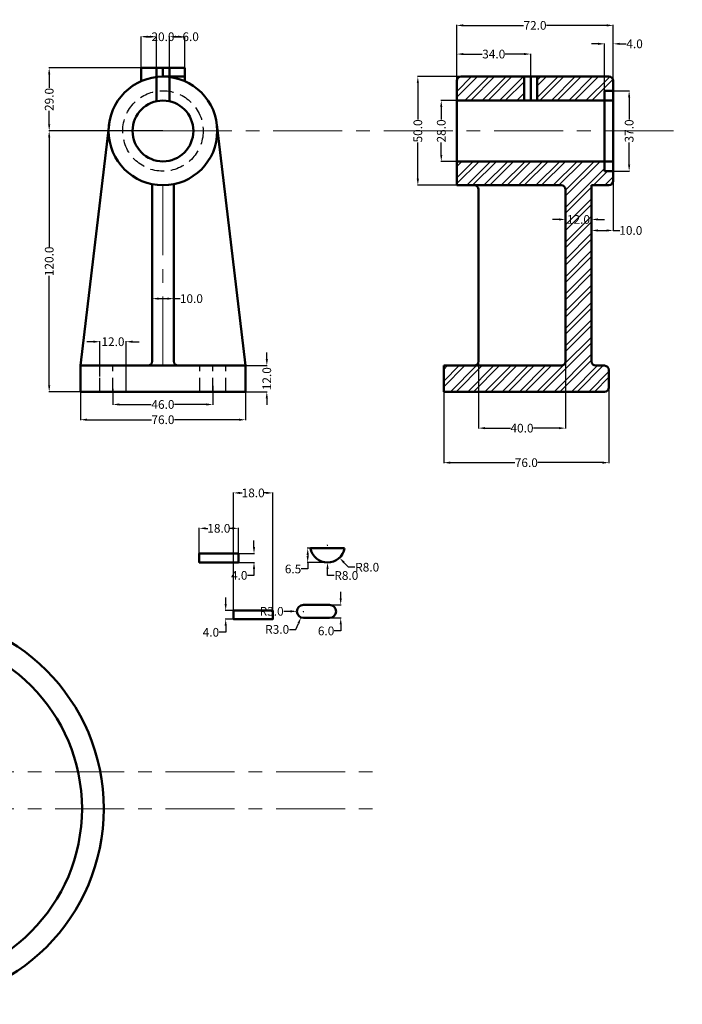
# Model space of a CAD drawing. Units: inches. Extents: x -30 to 602, y 452 to 930.
# Tile 3 of 3: x 297 to 602, y 452 to 905. Entities that reach past the tile are written whole.
import ezdxf

# ---------------------------------------------------------------- set-up
doc = ezdxf.new("R2010")
doc.units = ezdxf.units.IN
doc.header["$MEASUREMENT"] = 0
doc.linetypes.add('CENTER', pattern=[50.8, 31.75, -6.35, 6.35, -6.35])
doc.linetypes.add('HIDDEN', pattern=[9.525, 6.35, -3.175])
for name, color, linetype, lineweight in [('M-CNTR', 1, 'CENTER', 18), ('M-DIMS', 2, 'Continuous', 25), ('M-HATC', 8, 'Continuous', 18), ('M-HIDN', 6, 'HIDDEN', 25), ('M-OUTL', 7, 'Continuous', 50)]:
    doc.layers.add(name, color=color, linetype=linetype, lineweight=lineweight)
doc.styles.get("Standard").update_dxf_attribs({"font": 'arial.ttf'})
doc.dimstyles.get("Standard").update_dxf_attribs({"dimtxt": 4, "dimasz": 3, "dimexe": 0.18, "dimexo": 0.0625, "dimgap": 0.09, "dimtad": 0, "dimtoh": 1, "dimdec": 1, "dimzin": 0, "dimdsep": 46, "dimtxsty": 'Standard', "dimcen": 0.09, "dimadec": 0, "dimazin": 0, "dimtfac": 1, "dimtdec": 1, "dimtofl": 0, "dimtmove": 0, "dimatfit": 3, "dimfxl": 1, "dimtolj": 1, "dimtzin": 0, "dimarcsym": 0})

# ---------------------------------------------------------------- blocks, each defined once
blk = doc.blocks.new('*D16')
at = {"layer": 'Defpoints', "color": 0, "transparency": 16777216}
for p in [(395.82, 745.65), (395.82, 733.65), (410.52, 733.65)]:
    blk.add_point(p, dxfattribs=at)
at = {"layer": 'M-DIMS', "color": 0, "lineweight": -2, "transparency": 16777216}
for p, q in [((410.52, 748.65), (410.52, 751.65)), ((395.88, 745.65), (410.7, 745.65)), ((395.88, 733.65), (410.7, 733.65)), ((410.52, 730.65), (410.52, 727.65))]:
    blk.add_line(p, q, dxfattribs=at)
at = {"layer": 'M-DIMS', "color": 0, "transparency": 16777216}
for points in [[(410.02, 748.65), (411.02, 748.65), (410.52, 745.65)], [(410.02, 730.65), (411.02, 730.65), (410.52, 733.65)]]:
    blk.add_solid(points, dxfattribs=at)
at = {"layer": 'M-DIMS', "color": 0, "transparency": 16777216, "insert": (410.52, 739.65), "char_height": 4, "attachment_point": 5, "rotation": 90}
blk.add_mtext('\\A1;12.0', dxfattribs=at)
blk = doc.blocks.new('*D17')
at = {"layer": 'Defpoints', "color": 0, "transparency": 16777216}
for p in [(367.72, 776.49), (357.72, 770.92), (367.72, 770.92)]:
    blk.add_point(p, dxfattribs=at)
at = {"layer": 'M-DIMS', "color": 0, "lineweight": -2, "transparency": 16777216}
for p, q in [((357.72, 770.98), (357.72, 776.67)), ((360.72, 776.49), (364.72, 776.49)), ((367.72, 770.98), (367.72, 776.67)), ((367.72, 776.49), (370.72, 776.49))]:
    blk.add_line(p, q, dxfattribs=at)
at = {"layer": 'M-DIMS', "color": 0, "transparency": 16777216}
for points in [[(360.72, 776.99), (360.72, 775.99), (357.72, 776.49)], [(364.72, 776.99), (364.72, 775.99), (367.72, 776.49)]]:
    blk.add_solid(points, dxfattribs=at)
at = {"layer": 'M-DIMS', "color": 0, "transparency": 16777216, "insert": (375.81, 776.49), "char_height": 4, "attachment_point": 5}
blk.add_mtext('\\A1;10.0', dxfattribs=at)
blk = doc.blocks.new('*D18')
at = {"layer": 'Defpoints', "color": 0, "transparency": 16777216}
for p in [(345.72, 756.67), (333.72, 740.57), (345.72, 739.65)]:
    blk.add_point(p, dxfattribs=at)
at = {"layer": 'M-DIMS', "color": 0, "lineweight": -2, "transparency": 16777216}
for p, q in [((330.72, 756.67), (327.72, 756.67)), ((333.72, 740.63), (333.72, 756.85)), ((345.72, 739.71), (345.72, 756.85)), ((348.72, 756.67), (351.72, 756.67))]:
    blk.add_line(p, q, dxfattribs=at)
at = {"layer": 'M-DIMS', "color": 0, "transparency": 16777216}
for points in [[(330.72, 757.17), (330.72, 756.17), (333.72, 756.67)], [(348.72, 757.17), (348.72, 756.17), (345.72, 756.67)]]:
    blk.add_solid(points, dxfattribs=at)
at = {"layer": 'M-DIMS', "color": 0, "transparency": 16777216, "insert": (339.72, 756.67), "char_height": 4, "attachment_point": 5}
blk.add_mtext('\\A1;12.0', dxfattribs=at)
blk = doc.blocks.new('*D19')
at = {"layer": 'Defpoints', "color": 0, "transparency": 16777216}
for p in [(339.72, 735.01), (385.72, 736.37), (385.72, 727.79)]:
    blk.add_point(p, dxfattribs=at)
at = {"layer": 'M-DIMS', "color": 0, "lineweight": -2, "transparency": 16777216}
for p, q in [((339.72, 734.94), (339.72, 727.61)), ((385.72, 736.31), (385.72, 727.61)), ((342.72, 727.79), (357.37, 727.79)), ((382.72, 727.79), (368.08, 727.79))]:
    blk.add_line(p, q, dxfattribs=at)
at = {"layer": 'M-DIMS', "color": 0, "transparency": 16777216}
for points in [[(342.72, 728.29), (342.72, 727.29), (339.72, 727.79)], [(382.72, 728.29), (382.72, 727.29), (385.72, 727.79)]]:
    blk.add_solid(points, dxfattribs=at)
at = {"layer": 'M-DIMS', "color": 0, "transparency": 16777216, "insert": (362.72, 727.79), "char_height": 4, "attachment_point": 5}
blk.add_mtext('\\A1;46.0', dxfattribs=at)
blk = doc.blocks.new('*D20')
at = {"layer": 'Defpoints', "color": 0, "transparency": 16777216}
for p in [(324.72, 733.65), (400.72, 733.65), (400.72, 720.77)]:
    blk.add_point(p, dxfattribs=at)
at = {"layer": 'M-DIMS', "color": 0, "lineweight": -2, "transparency": 16777216}
for p, q in [((324.72, 733.59), (324.72, 720.59)), ((400.72, 733.59), (400.72, 720.59)), ((327.72, 720.77), (357.46, 720.77)), ((397.72, 720.77), (367.99, 720.77))]:
    blk.add_line(p, q, dxfattribs=at)
at = {"layer": 'M-DIMS', "color": 0, "transparency": 16777216}
for points in [[(327.72, 721.27), (327.72, 720.27), (324.72, 720.77)], [(397.72, 721.27), (397.72, 720.27), (400.72, 720.77)]]:
    blk.add_solid(points, dxfattribs=at)
at = {"layer": 'M-DIMS', "color": 0, "transparency": 16777216, "insert": (362.72, 720.77), "char_height": 4, "attachment_point": 5}
blk.add_mtext('\\A1;76.0', dxfattribs=at)
blk = doc.blocks.new('*D21')
at = {"layer": 'Defpoints', "color": 0, "transparency": 16777216}
for p in [(569.95, 902.22), (497.95, 865.23), (569.95, 860.94)]:
    blk.add_point(p, dxfattribs=at)
at = {"layer": 'M-DIMS', "color": 0, "lineweight": -2, "transparency": 16777216}
for p, q in [((497.95, 865.29), (497.95, 902.4)), ((500.95, 902.22), (528.69, 902.22)), ((566.95, 902.22), (539.22, 902.22)), ((569.95, 861), (569.95, 902.4))]:
    blk.add_line(p, q, dxfattribs=at)
at = {"layer": 'M-DIMS', "color": 0, "transparency": 16777216}
for points in [[(500.95, 902.72), (500.95, 901.72), (497.95, 902.22)], [(566.95, 902.72), (566.95, 901.72), (569.95, 902.22)]]:
    blk.add_solid(points, dxfattribs=at)
at = {"layer": 'M-DIMS', "color": 0, "transparency": 16777216, "insert": (533.95, 902.22), "char_height": 4, "attachment_point": 5}
blk.add_mtext('\\A1;72.0', dxfattribs=at)
blk = doc.blocks.new('*D22')
at = {"layer": 'Defpoints', "color": 0, "transparency": 16777216}
for p in [(497.95, 889.02), (497.95, 873.15), (531.95, 873.15)]:
    blk.add_point(p, dxfattribs=at)
at = {"layer": 'M-DIMS', "color": 0, "lineweight": -2, "transparency": 16777216}
for p, q in [((497.95, 873.21), (497.95, 889.2)), ((500.95, 889.02), (509.68, 889.02)), ((528.95, 889.02), (520.23, 889.02)), ((531.95, 873.21), (531.95, 889.2))]:
    blk.add_line(p, q, dxfattribs=at)
at = {"layer": 'M-DIMS', "color": 0, "transparency": 16777216}
for points in [[(500.95, 889.52), (500.95, 888.52), (497.95, 889.02)], [(528.95, 889.52), (528.95, 888.52), (531.95, 889.02)]]:
    blk.add_solid(points, dxfattribs=at)
at = {"layer": 'M-DIMS', "color": 0, "transparency": 16777216, "insert": (514.95, 889.02), "char_height": 4, "attachment_point": 5}
blk.add_mtext('\\A1;34.0', dxfattribs=at)
blk = doc.blocks.new('*D23')
at = {"layer": 'Defpoints', "color": 0, "transparency": 16777216}
for p in [(569.95, 893.73), (569.95, 861.83), (565.95, 860.76)]:
    blk.add_point(p, dxfattribs=at)
at = {"layer": 'M-DIMS', "color": 0, "lineweight": -2, "transparency": 16777216}
for p, q in [((562.95, 893.73), (559.95, 893.73)), ((565.95, 860.82), (565.95, 893.91)), ((569.95, 861.89), (569.95, 893.91)), ((572.95, 893.73), (575.95, 893.73))]:
    blk.add_line(p, q, dxfattribs=at)
at = {"layer": 'M-DIMS', "color": 0, "transparency": 16777216}
for points in [[(562.95, 894.23), (562.95, 893.23), (565.95, 893.73)], [(572.95, 894.23), (572.95, 893.23), (569.95, 893.73)]]:
    blk.add_solid(points, dxfattribs=at)
at = {"layer": 'M-DIMS', "color": 0, "transparency": 16777216, "insert": (579.76, 893.73), "char_height": 4, "attachment_point": 5}
blk.add_mtext('\\A1;4.0', dxfattribs=at)
blk = doc.blocks.new('*D24')
at = {"layer": 'Defpoints', "color": 0, "transparency": 16777216}
for p in [(569.95, 872.15), (569.95, 835.15), (577.26, 835.15)]:
    blk.add_point(p, dxfattribs=at)
at = {"layer": 'M-DIMS', "color": 0, "lineweight": -2, "transparency": 16777216}
for p, q in [((570.02, 872.15), (577.44, 872.15)), ((577.26, 869.15), (577.26, 858.93)), ((577.26, 838.15), (577.26, 848.37)), ((570.02, 835.15), (577.44, 835.15))]:
    blk.add_line(p, q, dxfattribs=at)
at = {"layer": 'M-DIMS', "color": 0, "transparency": 16777216}
for points in [[(576.76, 869.15), (577.76, 869.15), (577.26, 872.15)], [(576.76, 838.15), (577.76, 838.15), (577.26, 835.15)]]:
    blk.add_solid(points, dxfattribs=at)
at = {"layer": 'M-DIMS', "color": 0, "transparency": 16777216, "insert": (577.26, 853.65), "char_height": 4, "attachment_point": 5, "rotation": 90}
blk.add_mtext('\\A1;37.0', dxfattribs=at)
blk = doc.blocks.new('*D25')
at = {"layer": 'Defpoints', "color": 0, "transparency": 16777216}
for p in [(501.37, 867.65), (490.8, 839.65), (501.37, 839.65)]:
    blk.add_point(p, dxfattribs=at)
at = {"layer": 'M-DIMS', "color": 0, "lineweight": -2, "transparency": 16777216}
for p, q in [((501.3, 867.65), (490.62, 867.65)), ((490.8, 864.65), (490.8, 858.96)), ((490.8, 842.65), (490.8, 848.34)), ((501.3, 839.65), (490.62, 839.65))]:
    blk.add_line(p, q, dxfattribs=at)
at = {"layer": 'M-DIMS', "color": 0, "transparency": 16777216}
for points in [[(490.3, 864.65), (491.3, 864.65), (490.8, 867.65)], [(490.3, 842.65), (491.3, 842.65), (490.8, 839.65)]]:
    blk.add_solid(points, dxfattribs=at)
at = {"layer": 'M-DIMS', "color": 0, "transparency": 16777216, "insert": (490.8, 853.65), "char_height": 4, "attachment_point": 5, "rotation": 90}
blk.add_mtext('\\A1;28.0', dxfattribs=at)
blk = doc.blocks.new('*D26')
at = {"layer": 'Defpoints', "color": 0, "transparency": 16777216}
for p in [(502.42, 878.65), (480.02, 828.65), (499.89, 828.65)]:
    blk.add_point(p, dxfattribs=at)
at = {"layer": 'M-DIMS', "color": 0, "lineweight": -2, "transparency": 16777216}
for p, q in [((502.36, 878.65), (479.84, 878.65)), ((480.02, 875.65), (480.02, 858.93)), ((480.02, 831.65), (480.02, 848.37)), ((499.82, 828.65), (479.84, 828.65))]:
    blk.add_line(p, q, dxfattribs=at)
at = {"layer": 'M-DIMS', "color": 0, "transparency": 16777216}
for points in [[(479.52, 875.65), (480.52, 875.65), (480.02, 878.65)], [(479.52, 831.65), (480.52, 831.65), (480.02, 828.65)]]:
    blk.add_solid(points, dxfattribs=at)
at = {"layer": 'M-DIMS', "color": 0, "transparency": 16777216, "insert": (480.02, 853.65), "char_height": 4, "attachment_point": 5, "rotation": 90}
blk.add_mtext('\\A1;50.0', dxfattribs=at)
blk = doc.blocks.new('*D27')
at = {"layer": 'Defpoints', "color": 0, "transparency": 16777216}
for p in [(547.95, 812.93), (559.95, 812.93), (559.95, 811.58)]:
    blk.add_point(p, dxfattribs=at)
at = {"layer": 'M-DIMS', "color": 0, "lineweight": -2, "transparency": 16777216}
for p, q in [((544.95, 812.93), (541.95, 812.93)), ((547.95, 812.99), (547.95, 813.11)), ((559.95, 811.64), (559.95, 813.11)), ((562.95, 812.93), (565.95, 812.93))]:
    blk.add_line(p, q, dxfattribs=at)
at = {"layer": 'M-DIMS', "color": 0, "transparency": 16777216}
for points in [[(544.95, 813.43), (544.95, 812.43), (547.95, 812.93)], [(562.95, 813.43), (562.95, 812.43), (559.95, 812.93)]]:
    blk.add_solid(points, dxfattribs=at)
at = {"layer": 'M-DIMS', "color": 0, "transparency": 16777216, "insert": (553.95, 812.93), "char_height": 4, "attachment_point": 5}
blk.add_mtext('\\A1;12.0', dxfattribs=at)
blk = doc.blocks.new('*D28')
at = {"layer": 'Defpoints', "color": 0, "transparency": 16777216}
for p in [(569.95, 835.15), (559.95, 823.74), (569.95, 807.86)]:
    blk.add_point(p, dxfattribs=at)
at = {"layer": 'M-DIMS', "color": 0, "lineweight": -2, "transparency": 16777216}
for p, q in [((569.95, 835.09), (569.95, 807.68)), ((559.95, 823.67), (559.95, 807.68)), ((562.95, 807.86), (566.95, 807.86)), ((569.95, 807.86), (572.95, 807.86))]:
    blk.add_line(p, q, dxfattribs=at)
at = {"layer": 'M-DIMS', "color": 0, "transparency": 16777216}
for points in [[(562.95, 808.36), (562.95, 807.36), (559.95, 807.86)], [(566.95, 808.36), (566.95, 807.36), (569.95, 807.86)]]:
    blk.add_solid(points, dxfattribs=at)
at = {"layer": 'M-DIMS', "color": 0, "transparency": 16777216, "insert": (578.04, 807.86), "char_height": 4, "attachment_point": 5}
blk.add_mtext('\\A1;10.0', dxfattribs=at)
blk = doc.blocks.new('*D29')
at = {"layer": 'Defpoints', "color": 0, "transparency": 16777216}
for p in [(491.95, 739.65), (567.95, 741.21), (567.95, 701.02)]:
    blk.add_point(p, dxfattribs=at)
at = {"layer": 'M-DIMS', "color": 0, "lineweight": -2, "transparency": 16777216}
for p, q in [((491.95, 739.59), (491.95, 700.84)), ((567.95, 741.15), (567.95, 700.84)), ((494.95, 701.02), (524.69, 701.02)), ((564.95, 701.02), (535.22, 701.02))]:
    blk.add_line(p, q, dxfattribs=at)
at = {"layer": 'M-DIMS', "color": 0, "transparency": 16777216}
for points in [[(494.95, 701.52), (494.95, 700.52), (491.95, 701.02)], [(564.95, 701.52), (564.95, 700.52), (567.95, 701.02)]]:
    blk.add_solid(points, dxfattribs=at)
at = {"layer": 'M-DIMS', "color": 0, "transparency": 16777216, "insert": (529.95, 701.02), "char_height": 4, "attachment_point": 5}
blk.add_mtext('\\A1;76.0', dxfattribs=at)
blk = doc.blocks.new('*D30')
at = {"layer": 'Defpoints', "color": 0, "transparency": 16777216}
for p in [(507.95, 764.86), (547.95, 764.86), (547.95, 716.9)]:
    blk.add_point(p, dxfattribs=at)
at = {"layer": 'M-DIMS', "color": 0, "lineweight": -2, "transparency": 16777216}
for p, q in [((507.95, 764.79), (507.95, 716.72)), ((547.95, 764.79), (547.95, 716.72)), ((510.95, 716.9), (522.59, 716.9)), ((544.95, 716.9), (533.31, 716.9))]:
    blk.add_line(p, q, dxfattribs=at)
at = {"layer": 'M-DIMS', "color": 0, "transparency": 16777216}
for points in [[(510.95, 717.4), (510.95, 716.4), (507.95, 716.9)], [(544.95, 717.4), (544.95, 716.4), (547.95, 716.9)]]:
    blk.add_solid(points, dxfattribs=at)
at = {"layer": 'M-DIMS', "color": 0, "transparency": 16777216, "insert": (527.95, 716.9), "char_height": 4, "attachment_point": 5}
blk.add_mtext('\\A1;40.0', dxfattribs=at)
blk = doc.blocks.new('*D44')
at = {"layer": 'Defpoints', "color": 0, "transparency": 16777216}
for p in [(397.44, 670.8), (379.44, 657.76), (397.44, 657.15)]:
    blk.add_point(p, dxfattribs=at)
at = {"layer": 'M-DIMS', "color": 0, "lineweight": -2, "transparency": 16777216}
for p, q in [((379.44, 657.82), (379.44, 670.98)), ((382.44, 670.8), (383.35, 670.8)), ((394.44, 670.8), (393.53, 670.8)), ((397.44, 657.22), (397.44, 670.98))]:
    blk.add_line(p, q, dxfattribs=at)
at = {"layer": 'M-DIMS', "color": 0, "transparency": 16777216}
for points in [[(382.44, 671.3), (382.44, 670.3), (379.44, 670.8)], [(394.44, 671.3), (394.44, 670.3), (397.44, 670.8)]]:
    blk.add_solid(points, dxfattribs=at)
at = {"layer": 'M-DIMS', "color": 0, "transparency": 16777216, "insert": (388.44, 670.8), "char_height": 4, "attachment_point": 5}
blk.add_mtext('\\A1;18.0', dxfattribs=at)
blk = doc.blocks.new('*D45')
at = {"layer": 'Defpoints', "color": 0, "transparency": 16777216}
for p in [(397.44, 659.15), (397.44, 655.15), (404.62, 655.15)]:
    blk.add_point(p, dxfattribs=at)
at = {"layer": 'M-DIMS', "color": 0, "lineweight": -2, "transparency": 16777216}
for p, q in [((404.62, 662.15), (404.62, 665.15)), ((397.5, 659.15), (404.8, 659.15)), ((397.5, 655.15), (404.8, 655.15)), ((404.62, 649.15), (401.62, 649.15)), ((404.62, 652.15), (404.62, 649.15))]:
    blk.add_line(p, q, dxfattribs=at)
at = {"layer": 'M-DIMS', "color": 0, "transparency": 16777216}
for points in [[(404.12, 662.15), (405.12, 662.15), (404.62, 659.15)], [(404.12, 652.15), (405.12, 652.15), (404.62, 655.15)]]:
    blk.add_solid(points, dxfattribs=at)
at = {"layer": 'M-DIMS', "color": 0, "transparency": 16777216, "insert": (397.81, 649.15), "char_height": 4, "attachment_point": 5}
blk.add_mtext('\\A1;4.0', dxfattribs=at)
blk = doc.blocks.new('*D46')
at = {"layer": 'Defpoints', "color": 0, "transparency": 16777216}
for p in [(438.46, 663.1), (443.95, 657.28)]:
    blk.add_point(p, dxfattribs=at)
at = {"layer": 'M-DIMS', "color": 0, "lineweight": -2, "transparency": 16777216}
for p, q in [((438.37, 663.1), (438.55, 663.1)), ((438.46, 663.01), (438.46, 663.19)), ((448.07, 652.92), (446.01, 655.1)), ((451.07, 652.92), (448.07, 652.92))]:
    blk.add_line(p, q, dxfattribs=at)
at = {"layer": 'M-DIMS', "color": 0, "transparency": 16777216}
blk.add_solid([(446.37, 655.44), (445.65, 654.76), (443.95, 657.28)], dxfattribs=at)
at = {"layer": 'M-DIMS', "color": 0, "transparency": 16777216, "insert": (456.71, 652.92), "char_height": 4, "attachment_point": 5}
blk.add_mtext('\\A1;R8.0', dxfattribs=at)
blk = doc.blocks.new('*D47')
at = {"layer": 'Defpoints', "color": 0, "transparency": 16777216}
for p in [(438.46, 661.6), (429.34, 655.1), (438.46, 655.1)]:
    blk.add_point(p, dxfattribs=at)
at = {"layer": 'M-DIMS', "color": 0, "lineweight": -2, "transparency": 16777216}
for p, q in [((438.4, 661.6), (429.16, 661.6)), ((429.34, 658.6), (429.34, 658.1)), ((438.4, 655.1), (429.16, 655.1)), ((429.34, 655.1), (429.34, 652.1)), ((429.34, 652.1), (426.34, 652.1))]:
    blk.add_line(p, q, dxfattribs=at)
at = {"layer": 'M-DIMS', "color": 0, "transparency": 16777216}
for points in [[(428.84, 658.6), (429.84, 658.6), (429.34, 661.6)], [(428.84, 658.1), (429.84, 658.1), (429.34, 655.1)]]:
    blk.add_solid(points, dxfattribs=at)
at = {"layer": 'M-DIMS', "color": 0, "transparency": 16777216, "insert": (422.59, 652.1), "char_height": 4, "attachment_point": 5}
blk.add_mtext('\\A1;6.5', dxfattribs=at)
blk = doc.blocks.new('*D48')
at = {"layer": 'Defpoints', "color": 0, "transparency": 16777216}
for p in [(395.24, 632.97), (391.59, 628.97), (395.24, 628.97)]:
    blk.add_point(p, dxfattribs=at)
at = {"layer": 'M-DIMS', "color": 0, "lineweight": -2, "transparency": 16777216}
for p, q in [((391.59, 635.97), (391.59, 638.97)), ((395.17, 632.97), (391.41, 632.97)), ((395.17, 628.97), (391.41, 628.97)), ((391.59, 625.97), (391.59, 622.97)), ((391.59, 622.97), (388.59, 622.97))]:
    blk.add_line(p, q, dxfattribs=at)
at = {"layer": 'M-DIMS', "color": 0, "transparency": 16777216}
for points in [[(391.09, 635.97), (392.09, 635.97), (391.59, 632.97)], [(391.09, 625.97), (392.09, 625.97), (391.59, 628.97)]]:
    blk.add_solid(points, dxfattribs=at)
at = {"layer": 'M-DIMS', "color": 0, "transparency": 16777216, "insert": (384.79, 622.97), "char_height": 4, "attachment_point": 5}
blk.add_mtext('\\A1;4.0', dxfattribs=at)
blk = doc.blocks.new('*D49')
at = {"layer": 'Defpoints', "color": 0, "transparency": 16777216}
for p in [(433.07, 635.59), (433.07, 629.59), (444.53, 629.59)]:
    blk.add_point(p, dxfattribs=at)
at = {"layer": 'M-DIMS', "color": 0, "lineweight": -2, "transparency": 16777216}
for p, q in [((444.53, 638.59), (444.53, 641.59)), ((433.13, 635.59), (444.71, 635.59)), ((433.13, 629.59), (444.71, 629.59)), ((444.53, 626.59), (444.53, 623.59)), ((444.53, 623.59), (441.53, 623.59))]:
    blk.add_line(p, q, dxfattribs=at)
at = {"layer": 'M-DIMS', "color": 0, "transparency": 16777216}
for points in [[(444.03, 638.59), (445.03, 638.59), (444.53, 635.59)], [(444.03, 626.59), (445.03, 626.59), (444.53, 629.59)]]:
    blk.add_solid(points, dxfattribs=at)
at = {"layer": 'M-DIMS', "color": 0, "transparency": 16777216, "insert": (437.79, 623.59), "char_height": 4, "attachment_point": 5}
blk.add_mtext('\\A1;6.0', dxfattribs=at)
blk = doc.blocks.new('*D50')
at = {"layer": 'Defpoints', "color": 0, "transparency": 16777216}
for p in [(426.24, 629.83), (427.39, 632.59)]:
    blk.add_point(p, dxfattribs=at)
at = {"layer": 'M-DIMS', "color": 0, "lineweight": -2, "transparency": 16777216}
for p, q in [((427.3, 632.59), (427.48, 632.59)), ((427.39, 632.5), (427.39, 632.68)), ((423.92, 624.29), (425.08, 627.06)), ((420.92, 624.29), (423.92, 624.29))]:
    blk.add_line(p, q, dxfattribs=at)
at = {"layer": 'M-DIMS', "color": 0, "transparency": 16777216}
blk.add_solid([(424.62, 627.25), (425.54, 626.87), (426.24, 629.83)], dxfattribs=at)
at = {"layer": 'M-DIMS', "color": 0, "transparency": 16777216, "insert": (415.29, 624.29), "char_height": 4, "attachment_point": 5}
blk.add_mtext('\\A1;R3.0', dxfattribs=at)
blk = doc.blocks.new('*D58')
at = {"layer": 'Defpoints', "color": 0, "transparency": 16777216}
for p in [(310.37, 853.65), (362.72, 853.65), (324.72, 733.65)]:
    blk.add_point(p, dxfattribs=at)
at = {"layer": 'M-DIMS', "color": 0, "lineweight": -2, "transparency": 16777216}
for p, q in [((362.66, 853.65), (310.19, 853.65)), ((310.37, 850.65), (310.37, 800.29)), ((310.37, 736.65), (310.37, 787.01)), ((324.66, 733.65), (310.19, 733.65))]:
    blk.add_line(p, q, dxfattribs=at)
at = {"layer": 'M-DIMS', "color": 0, "transparency": 16777216}
for points in [[(309.87, 850.65), (310.87, 850.65), (310.37, 853.65)], [(309.87, 736.65), (310.87, 736.65), (310.37, 733.65)]]:
    blk.add_solid(points, dxfattribs=at)
at = {"layer": 'M-DIMS', "color": 0, "transparency": 16777216, "insert": (310.37, 793.65), "char_height": 4, "attachment_point": 5, "rotation": 90}
blk.add_mtext('\\A1;120.0', dxfattribs=at)
blk = doc.blocks.new('*D59')
at = {"layer": 'Defpoints', "color": 0, "transparency": 16777216}
for p in [(310.37, 882.65), (352.72, 882.65), (362.72, 853.65)]:
    blk.add_point(p, dxfattribs=at)
at = {"layer": 'M-DIMS', "color": 0, "lineweight": -2, "transparency": 16777216}
for p, q in [((352.66, 882.65), (310.19, 882.65)), ((310.37, 879.65), (310.37, 873.46)), ((310.37, 856.65), (310.37, 862.84)), ((362.66, 853.65), (310.19, 853.65))]:
    blk.add_line(p, q, dxfattribs=at)
at = {"layer": 'M-DIMS', "color": 0, "transparency": 16777216}
for points in [[(309.87, 879.65), (310.87, 879.65), (310.37, 882.65)], [(309.87, 856.65), (310.87, 856.65), (310.37, 853.65)]]:
    blk.add_solid(points, dxfattribs=at)
at = {"layer": 'M-DIMS', "color": 0, "transparency": 16777216, "insert": (310.37, 868.15), "char_height": 4, "attachment_point": 5, "rotation": 90}
blk.add_mtext('\\A1;29.0', dxfattribs=at)
blk = doc.blocks.new('*D60')
at = {"layer": 'Defpoints', "color": 0, "transparency": 16777216}
for p in [(372.72, 897), (352.72, 882.65), (372.72, 882.65)]:
    blk.add_point(p, dxfattribs=at)
at = {"layer": 'M-DIMS', "color": 0, "lineweight": -2, "transparency": 16777216}
for p, q in [((352.72, 882.71), (352.72, 897.18)), ((372.72, 882.71), (372.72, 897.18)), ((355.72, 897), (357.41, 897)), ((369.72, 897), (368.04, 897))]:
    blk.add_line(p, q, dxfattribs=at)
at = {"layer": 'M-DIMS', "color": 0, "transparency": 16777216}
for points in [[(355.72, 897.5), (355.72, 896.5), (352.72, 897)], [(369.72, 897.5), (369.72, 896.5), (372.72, 897)]]:
    blk.add_solid(points, dxfattribs=at)
at = {"layer": 'M-DIMS', "color": 0, "transparency": 16777216, "insert": (362.72, 897), "char_height": 4, "attachment_point": 5}
blk.add_mtext('\\A1;20.0', dxfattribs=at)
blk = doc.blocks.new('*D61')
at = {"layer": 'Defpoints', "color": 0, "transparency": 16777216}
for p in [(365.72, 897), (359.72, 882.65), (365.72, 882.65)]:
    blk.add_point(p, dxfattribs=at)
at = {"layer": 'M-DIMS', "color": 0, "lineweight": -2, "transparency": 16777216}
for p, q in [((359.72, 882.71), (359.72, 897.18)), ((365.72, 882.71), (365.72, 897.18)), ((356.72, 897), (353.72, 897)), ((368.72, 897), (371.72, 897))]:
    blk.add_line(p, q, dxfattribs=at)
at = {"layer": 'M-DIMS', "color": 0, "transparency": 16777216}
for points in [[(356.72, 897.5), (356.72, 896.5), (359.72, 897)], [(368.72, 897.5), (368.72, 896.5), (365.72, 897)]]:
    blk.add_solid(points, dxfattribs=at)
at = {"layer": 'M-DIMS', "color": 0, "transparency": 16777216, "insert": (375.46, 897), "char_height": 4, "attachment_point": 5}
blk.add_mtext('\\A1;6.0', dxfattribs=at)
blk = doc.blocks.new('*D62')
at = {"layer": 'Defpoints', "color": 0, "transparency": 16777216}
for p in [(413.237044, 687.097154), (395.237044, 632.969264), (413.237044, 632.969264)]:
    blk.add_point(p, dxfattribs=at)
at = {"layer": 'M-DIMS', "color": 0, "lineweight": -2, "transparency": 16777216}
for p, q in [((395.237044, 633.031764), (395.237044, 687.277154)), ((398.237044, 687.097154), (399.147044, 687.097154)), ((410.237044, 687.097154), (409.327044, 687.097154)), ((413.237044, 633.031764), (413.237044, 687.277154))]:
    blk.add_line(p, q, dxfattribs=at)
at = {"layer": 'M-DIMS', "color": 0, "transparency": 16777216}
for points in [[(398.237044, 687.597154), (398.237044, 686.597154), (395.237044, 687.097154)], [(410.237044, 687.597154), (410.237044, 686.597154), (413.237044, 687.097154)]]:
    blk.add_solid(points, dxfattribs=at)
at = {"layer": 'M-DIMS', "color": 0, "transparency": 16777216, "insert": (404.237044, 687.097154), "char_height": 4, "attachment_point": 5}
blk.add_mtext('\\A1;18.0', dxfattribs=at)
blk = doc.blocks.new('*D68')
at = {"layer": 'Defpoints', "color": 0, "transparency": 16777216}
for p in [(438.46, 663.1), (438.46, 655.1)]:
    blk.add_point(p, dxfattribs=at)
at = {"layer": 'M-DIMS', "color": 0, "lineweight": -2, "transparency": 16777216}
for p, q in [((438.37, 663.1), (438.55, 663.1)), ((438.46, 663.01), (438.46, 663.19)), ((438.46, 649.1), (438.46, 652.1)), ((441.46, 649.1), (438.46, 649.1))]:
    blk.add_line(p, q, dxfattribs=at)
at = {"layer": 'M-DIMS', "color": 0, "transparency": 16777216}
blk.add_solid([(438.96, 652.1), (437.96, 652.1), (438.46, 655.1)], dxfattribs=at)
at = {"layer": 'M-DIMS', "color": 0, "transparency": 16777216, "insert": (447.1, 649.1), "char_height": 4, "attachment_point": 5}
blk.add_mtext('\\A1;R8.0', dxfattribs=at)
blk = doc.blocks.new('*D69')
at = {"layer": 'Defpoints', "color": 0, "transparency": 16777216}
for p in [(424.39, 632.6), (427.39, 632.59)]:
    blk.add_point(p, dxfattribs=at)
at = {"layer": 'M-DIMS', "color": 0, "lineweight": -2, "transparency": 16777216}
for p, q in [((418.39, 632.61), (421.39, 632.61)), ((427.3, 632.59), (427.48, 632.59)), ((427.39, 632.5), (427.39, 632.68))]:
    blk.add_line(p, q, dxfattribs=at)
at = {"layer": 'M-DIMS', "color": 0, "transparency": 16777216}
blk.add_solid([(421.39, 633.11), (421.39, 632.11), (424.39, 632.6)], dxfattribs=at)
at = {"layer": 'M-DIMS', "color": 0, "transparency": 16777216, "insert": (412.75, 632.61), "char_height": 4, "attachment_point": 5}
blk.add_mtext('\\A1;R3.0', dxfattribs=at)

msp = doc.modelspace()

# ---------------------------------------------------------------- hatches: boundary and pattern name
at = {"layer": 'M-HATC'}
h = msp.add_hatch(dxfattribs=at)
h.set_pattern_fill('ANSI32', color=256, scale=15)
h.paths.add_polyline_path([(528.95, 878.65), (499.95, 878.65, 0.414214), (497.95, 876.65), (497.95, 867.65), (528.95, 867.65)])
h.paths.add_polyline_path([(569.95, 876.65, 0.414214), (567.95, 878.65), (534.95, 878.65), (534.95, 867.65), (565.95, 867.65), (565.95, 872.15), (569.95, 872.15)])
h.paths.add_polyline_path([(559.95, 828.65), (567.95, 828.65, 0.414214), (569.95, 830.65), (569.95, 835.15), (565.95, 835.15), (565.95, 839.65), (497.95, 839.65), (497.95, 828.65), (545.95, 828.65, -0.414214), (547.95, 826.65), (547.95, 747.65, -0.414214), (545.95, 745.65), (491.95, 745.65), (491.95, 733.65), (565.95, 733.65, 0.414214), (567.95, 735.65), (567.95, 743.65, 0.414214), (565.95, 745.65), (561.95, 745.65, -0.414214), (559.95, 747.65)])

# ---------------------------------------------------------------- linework, layer by layer
at = {"layer": 'M-CNTR'}
for p, q in [((362.72, 853.65), (601.73, 853.65)), ((362.72, 745.65), (362.72, 828.65)), ((59.17, 558.79), (462.28, 558.79)), ((59.17, 541.79), (462.28, 541.79))]:
    msp.add_line(p, q, dxfattribs=at)
at = {"layer": 'M-HIDN'}
for p, q in [((333.72, 733.65), (333.72, 745.65)), ((339.72, 733.65), (339.72, 745.65)), ((345.72, 733.65), (345.72, 745.65)), ((379.72, 733.65), (379.72, 745.65)), ((385.72, 733.65), (385.72, 745.65)), ((391.72, 733.65), (391.72, 745.65))]:
    msp.add_line(p, q, dxfattribs=at)
msp.add_circle((362.72, 853.65), 18.5, dxfattribs=at)
at = {"layer": 'M-OUTL'}
for p, q in [((352.72, 882.65), (372.72, 882.65)), ((352.72, 876.56), (352.72, 882.65)), ((359.72, 867.33), (359.72, 882.65)), ((362.72, 878.65), (362.72, 882.65)), ((365.72, 867.33), (365.72, 882.65)), ((372.72, 876.56), (372.72, 882.65)), ((362.72, 878.65), (372.72, 878.65)), ((497.95, 876.65), (497.95, 828.65)), ((499.95, 878.65), (567.95, 878.65)), ((528.95, 878.65), (528.95, 867.65)), ((531.95, 878.65), (531.95, 867.65)), ((534.95, 878.65), (534.95, 867.65)), ((569.95, 876.65), (569.95, 830.65)), ((565.95, 872.15), (569.95, 872.15)), ((565.95, 872.15), (565.95, 835.15)), ((497.95, 867.65), (569.95, 867.65)), ((337.9, 856.6), (324.72, 745.65)), ((387.55, 856.6), (400.72, 745.65)), ((497.95, 839.65), (569.95, 839.65)), ((565.95, 835.15), (569.95, 835.15)), ((357.72, 747.65), (357.72, 829.16)), ((367.72, 747.65), (367.72, 829.16)), ((497.95, 828.65), (545.95, 828.65)), ((507.95, 826.65), (507.95, 747.65)), ((547.95, 826.65), (547.95, 747.65)), ((559.95, 828.65), (559.95, 747.65)), ((559.95, 828.65), (567.95, 828.65)), ((400.72, 745.65), (324.72, 745.65)), ((324.72, 745.65), (324.72, 733.65)), ((400.72, 733.65), (400.72, 745.65)), ((491.95, 745.65), (545.95, 745.65)), ((491.95, 733.65), (491.95, 745.65)), ((561.95, 745.65), (565.95, 745.65)), ((567.95, 743.65), (567.95, 735.65)), ((324.72, 733.65), (400.72, 733.65)), ((565.95, 733.65), (491.95, 733.65)), ((446.32, 661.6), (430.6, 661.6))]:
    msp.add_line(p, q, dxfattribs=at)
for points in [[(379.44, 659.15), (397.44, 659.15), (397.44, 655.15), (379.44, 655.15)], [(395.24, 632.97), (413.24, 632.97), (413.24, 628.97), (395.24, 628.97)]]:
    msp.add_lwpolyline(points, close=True, dxfattribs=at)
for points in [[(427.39, 635.59), (439.39, 635.59)], [(439.39, 629.59), (427.39, 629.59)]]:
    msp.add_lwpolyline(points, dxfattribs=at)
for centre, radius in [((362.72, 853.65), 25), ((362.72, 853.65), 14), ((245.47, 541.79), 90), ((245.47, 541.79), 80)]:
    msp.add_circle(centre, radius, dxfattribs=at)
for centre, radius, start, end in [((499.95, 876.65), 2, 90, 180), ((567.95, 876.65), 2, 0, 90), ((567.95, 830.65), 2, 270, 0), ((505.95, 826.65), 2, 0, 90), ((545.95, 826.65), 2, 0, 90), ((355.72, 747.65), 2, 270, 0), ((369.72, 747.65), 2, 180, 270), ((505.95, 747.65), 2, 270, 0), ((545.95, 747.65), 2, 270, 0), ((561.95, 747.65), 2, 180, 270), ((565.95, 743.65), 2, 0, 90), ((565.95, 735.65), 2, 270, 0), ((438.46, 663.1), 8, 190.8069, 349.1931), ((427.39, 632.59), 3, 90, 270), ((439.39, 632.59), 3, 270, 90)]:
    msp.add_arc(centre, radius, start, end, dxfattribs=at)

# ---------------------------------------------------------------- dimensions: what is measured, and where the dimension line sits
at = {"layer": 'M-DIMS'}
for base, p1, p2, override, picture, middle in [((569.95, 902.22), (497.95, 865.23), (569.95, 860.94), {"dimclrd": 0, "dimclre": 0, "dimclrt": 0}, '*D21', (533.95, 902.22)), ((372.72, 897), (352.72, 882.65), (372.72, 882.65), {"dimdec": 1, "dimlfac": 1, "dimrnd": 0, "dimzin": 0, "dimdsep": 46, "dimlunit": 2}, '*D60', (362.72, 897)), ((365.72, 897), (359.72, 882.65), (365.72, 882.65), {"dimdec": 1, "dimlfac": 1, "dimrnd": 0, "dimzin": 0, "dimdsep": 46, "dimlunit": 2}, '*D61', (375.46, 897)), ((569.95, 893.73), (565.95, 860.76), (569.95, 861.83), {"dimclrd": 0, "dimclre": 0, "dimclrt": 0}, '*D23', (579.76, 893.73)), ((497.95, 889.02), (531.95, 873.15), (497.95, 873.15), {"dimclrd": 0, "dimclre": 0, "dimclrt": 0}, '*D22', (514.95, 889.02)), ((569.95, 807.86), (559.95, 823.74), (569.95, 835.15), {"dimclrd": 0, "dimclre": 0, "dimclrt": 0}, '*D28', (578.04, 807.86)), ((559.95, 812.93), (547.95, 812.93), (559.95, 811.58), {"dimclrd": 0, "dimclre": 0, "dimclrt": 0}, '*D27', (553.95, 812.93)), ((367.72, 776.49), (357.72, 770.92), (367.72, 770.92), {"dimclrd": 0, "dimclre": 0, "dimclrt": 0}, '*D17', (375.81, 776.49)), ((547.95, 716.9), (507.95, 764.86), (547.95, 764.86), {"dimclrd": 0, "dimclre": 0, "dimclrt": 0}, '*D30', (527.95, 716.9)), ((345.72, 756.67), (333.72, 740.57), (345.72, 739.65), {"dimclrd": 0, "dimclre": 0, "dimclrt": 0}, '*D18', (339.72, 756.67)), ((567.95, 701.02), (491.95, 739.65), (567.95, 741.21), {"dimclrd": 0, "dimclre": 0, "dimclrt": 0}, '*D29', (529.95, 701.02)), ((385.72, 727.79), (339.72, 735.01), (385.72, 736.37), {"dimclrd": 0, "dimclre": 0, "dimclrt": 0}, '*D19', (362.72, 727.79)), ((400.72, 720.77), (324.72, 733.65), (400.72, 733.65), {"dimclrd": 0, "dimclre": 0, "dimclrt": 0}, '*D20', (362.72, 720.77)), ((413.24, 687.1), (395.24, 632.97), (413.24, 632.97), {"dimdec": 1, "dimlfac": 1, "dimrnd": 0, "dimzin": 0, "dimdsep": 46, "dimlunit": 2}, '*D62', (404.24, 687.1)), ((397.44, 670.8), (379.44, 657.76), (397.44, 657.15), {"dimclrd": 0, "dimclre": 0, "dimclrt": 0}, '*D44', (388.44, 670.8))]:
    dim = msp.add_linear_dim(base=base, p1=p1, p2=p2, dimstyle='Standard', override=override, dxfattribs=at)
    dim.commit()
    dim.dimension.update_dxf_attribs({"geometry": picture, "text_midpoint": middle})
for base, p1, p2, override, picture, middle in [((310.37, 882.65), (362.72, 853.65), (352.72, 882.65), {"dimdec": 1, "dimlfac": 1, "dimrnd": 0, "dimzin": 0, "dimdsep": 46, "dimlunit": 2}, '*D59', (310.37, 868.15)), ((480.02, 828.65), (502.42, 878.65), (499.89, 828.65), {"dimclrd": 0, "dimclre": 0, "dimclrt": 0}, '*D26', (480.02, 853.65)), ((577.26, 835.15), (569.95, 872.15), (569.95, 835.15), {"dimclrd": 0, "dimclre": 0, "dimclrt": 0}, '*D24', (577.26, 853.65)), ((490.8, 839.65), (501.37, 867.65), (501.37, 839.65), {"dimclrd": 0, "dimclre": 0, "dimclrt": 0}, '*D25', (490.8, 853.65)), ((310.37, 853.65), (324.72, 733.65), (362.72, 853.65), {"dimdec": 1, "dimlfac": 1, "dimrnd": 0, "dimzin": 0, "dimdsep": 46, "dimlunit": 2}, '*D58', (310.37, 793.65)), ((410.52, 733.65), (395.82, 745.65), (395.82, 733.65), {"dimclrd": 0, "dimclre": 0, "dimclrt": 0}, '*D16', (410.52, 739.65)), ((404.62, 655.15), (397.44, 659.15), (397.44, 655.15), {"dimclrd": 0, "dimclre": 0, "dimclrt": 0}, '*D45', (397.81, 649.15)), ((429.34, 655.1), (438.46, 661.6), (438.46, 655.1), {"dimclrd": 0, "dimclre": 0, "dimclrt": 0}, '*D47', (422.59, 652.1)), ((391.59, 628.97), (395.24, 632.97), (395.24, 628.97), {"dimclrd": 0, "dimclre": 0, "dimclrt": 0}, '*D48', (384.79, 622.97)), ((444.53, 629.59), (433.07, 635.59), (433.07, 629.59), {"dimclrd": 0, "dimclre": 0, "dimclrt": 0}, '*D49', (437.79, 623.59))]:
    dim = msp.add_linear_dim(base=base, p1=p1, p2=p2, angle=90, dimstyle='Standard', override=override, dxfattribs=at)
    dim.commit()
    dim.dimension.update_dxf_attribs({"geometry": picture, "text_midpoint": middle})
for center, mpoint, override, picture, middle in [((438.46, 663.1), (438.46, 655.1), {"dimdec": 1, "dimlfac": 1, "dimrnd": 0, "dimzin": 0, "dimdsep": 46, "dimlunit": 2}, '*D68', (447.1, 649.1)), ((438.46, 663.1), (443.95, 657.28), {"dimclrd": 0, "dimclre": 0, "dimclrt": 0}, '*D46', (456.71, 652.92)), ((427.39, 632.59), (424.39, 632.6), {"dimdec": 1, "dimlfac": 1, "dimrnd": 0, "dimzin": 0, "dimdsep": 46, "dimlunit": 2}, '*D69', (412.75, 632.61)), ((427.39, 632.59), (426.24, 629.83), {"dimclrd": 0, "dimclre": 0, "dimclrt": 0}, '*D50', (415.29, 624.29))]:
    dim = msp.add_radius_dim(center=center, mpoint=mpoint, dimstyle='Standard', override=override, dxfattribs=at)
    dim.commit()
    dim.dimension.update_dxf_attribs({"geometry": picture, "text_midpoint": middle})

doc.saveas('drawing.dxf')
